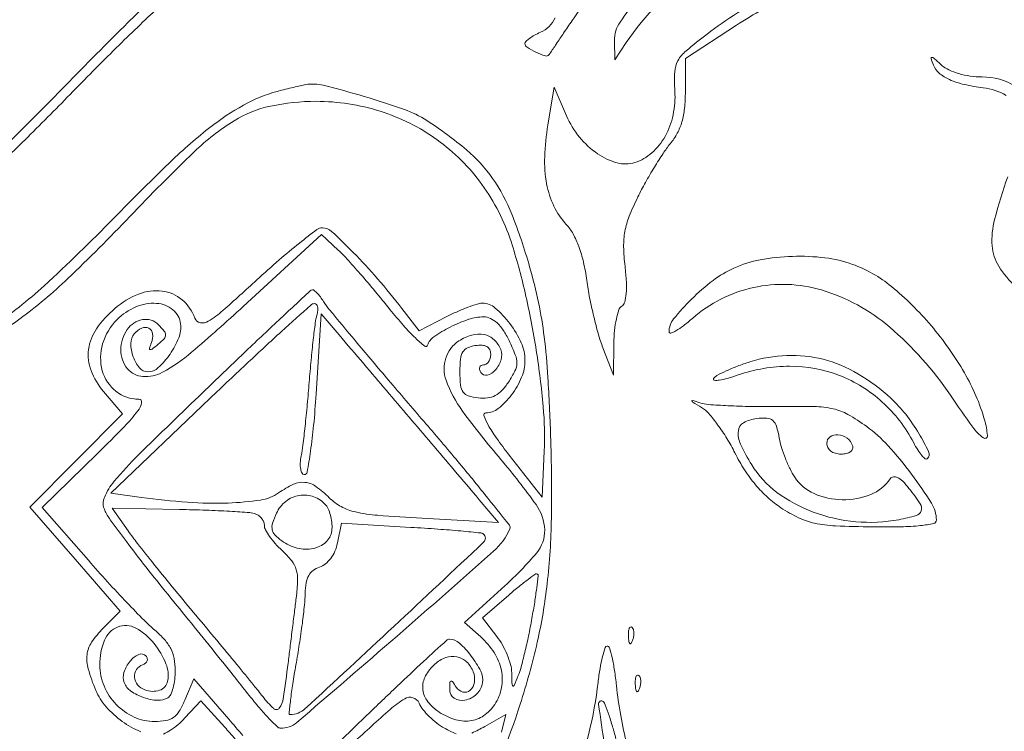
# Model space of a CAD drawing. Units: inches. Extents: x 2656 to 9931, y 1941 to 3068.
# Tile 37 of 46: x 2837 to 2847, y 2974 to 2981. Entities that reach past the tile are written whole.
import ezdxf

# ---------------------------------------------------------------- set-up
doc = ezdxf.new("R2010")
doc.units = ezdxf.units.IN
doc.layers.add('A-ANNO-DIMS', color=2, linetype='Continuous', lineweight=18)
doc.layers.add('A-ELEV-ORN', color=8, linetype='Continuous', lineweight=13)
doc.styles.get("Standard").update_dxf_attribs({"font": 'arial.ttf'})
doc.dimstyles.new('ISO-25', dxfattribs={"dimtxt": 6, "dimasz": 2.5, "dimexe": 1.25, "dimexo": 0.625, "dimtad": 1, "dimdec": 0, "dimlunit": 3, "dimtxsty": 'Standard', "dimcen": 2.5, "dimadec": 0, "dimazin": 0, "dimtfac": 1, "dimtdec": 0, "dimtmove": 0, "dimatfit": 3, "dimfxl": 1, "dimarcsym": 0})

# ---------------------------------------------------------------- blocks, each defined once
blk = doc.blocks.new('*D152')
at = {"layer": 'A-ANNO-DIMS', "color": 0, "lineweight": -2, "transparency": 16777216}
for p, q in [((2847.28, 2990.828), (2707.323, 2990.828)), ((2708.573, 2988.328), (2708.573, 2952.971)), ((2847.248, 2950.471), (2707.323, 2950.471))]:
    blk.add_line(p, q, dxfattribs=at)
at = {"layer": 'A-ANNO-DIMS', "color": 0, "transparency": 16777216}
for points in [[(2708.156, 2988.328), (2708.989, 2988.328), (2708.573, 2990.828)], [(2708.156, 2952.971), (2708.989, 2952.971), (2708.573, 2950.471)]]:
    blk.add_solid(points, dxfattribs=at)
at = {"layer": 'Defpoints', "color": 0, "transparency": 16777216}
for p in [(2847.905, 2990.828), (2708.573, 2950.471), (2847.873, 2950.471)]:
    blk.add_point(p, dxfattribs=at)
at = {"layer": 'A-ANNO-DIMS', "color": 0, "transparency": 16777216, "insert": (2704.843, 2970.649), "char_height": 6, "attachment_point": 5, "rotation": 90}
blk.add_mtext('3\'-4 1/2"', dxfattribs=at)
blk = doc.blocks.new('*D153')
at = {"layer": 'A-ANNO-DIMS', "color": 0, "lineweight": -2, "transparency": 16777216}
for p, q in [((2826.64, 2993.722), (2826.64, 2703.709)), ((2829.546, 2956.424), (2829.546, 2703.709)), ((2824.14, 2704.959), (2821.64, 2704.959)), ((2826.64, 2704.959), (2829.546, 2704.959)), ((2832.046, 2704.959), (2851.745, 2704.959))]:
    blk.add_line(p, q, dxfattribs=at)
at = {"layer": 'A-ANNO-DIMS', "color": 0, "transparency": 16777216}
for points in [[(2824.14, 2705.376), (2824.14, 2704.543), (2826.64, 2704.959)], [(2832.046, 2705.376), (2832.046, 2704.543), (2829.546, 2704.959)]]:
    blk.add_solid(points, dxfattribs=at)
at = {"layer": 'Defpoints', "color": 0, "transparency": 16777216}
for p in [(2826.64, 2994.347), (2829.546, 2957.049), (2829.546, 2704.959)]:
    blk.add_point(p, dxfattribs=at)
at = {"layer": 'A-ANNO-DIMS', "color": 0, "transparency": 16777216, "insert": (2843.145, 2708.65), "char_height": 6, "attachment_point": 5}
blk.add_mtext('0\'-3"', dxfattribs=at)
blk = doc.blocks.new('*D154')
at = {"layer": 'A-ANNO-DIMS', "color": 0, "lineweight": -2, "transparency": 16777216}
for p, q in [((2708.573, 2996.847), (2708.573, 2999.347)), ((2826.015, 2994.347), (2707.323, 2994.347)), ((2708.573, 2994.347), (2708.573, 2990.828)), ((2847.28, 2990.828), (2707.323, 2990.828)), ((2708.573, 2988.328), (2708.573, 2954.647))]:
    blk.add_line(p, q, dxfattribs=at)
at = {"layer": 'A-ANNO-DIMS', "color": 0, "transparency": 16777216}
for points in [[(2708.156, 2996.847), (2708.989, 2996.847), (2708.573, 2994.347)], [(2708.156, 2988.328), (2708.989, 2988.328), (2708.573, 2990.828)]]:
    blk.add_solid(points, dxfattribs=at)
at = {"layer": 'Defpoints', "color": 0, "transparency": 16777216}
for p in [(2826.64, 2994.347), (2708.573, 2990.828), (2847.905, 2990.828)]:
    blk.add_point(p, dxfattribs=at)
at = {"layer": 'A-ANNO-DIMS', "color": 0, "transparency": 16777216, "insert": (2704.843, 2970.237), "char_height": 6, "attachment_point": 5, "rotation": 90}
blk.add_mtext('0\'-3 1/2"', dxfattribs=at)

msp = doc.modelspace()

# ---------------------------------------------------------------- linework, layer by layer
at = {"layer": 'A-ELEV-ORN'}
for points in [[(2843.287, 2981.434, 0.03621), (2843.078, 2981.168, 0.154288), (2843.021, 2980.977), (2843.025, 2980.781), (2843.141, 2980.957, -0.10364), (2843.864, 2981.673, -0.058168)], [(2838.429, 2981.536, 0.015337), (2838.032, 2981.164, 0.003566), (2837.388, 2980.515, -0.006917), (2836.411, 2979.542, -0.058589)], [(2842.412, 2981.21, -0.182333), (2842.262, 2981.063, 0.022825), (2842.201, 2981.033, 0.031511), (2842.15, 2981.001, 0.032465), (2842.113, 2980.97, 0.205381), (2842.103, 2980.948, 0.258997), (2842.125, 2980.909, 0.02901), (2842.216, 2980.859, 0.028443), (2842.312, 2980.821, 0.331182), (2842.348, 2980.832, 0.005745), (2842.359, 2980.847, 0.000069), (2842.424, 2980.943, 0.000207), (2842.499, 2981.055, 0.000135), (2842.586, 2981.183, -0.032972), (2842.766, 2981.414, -0.024978)], [(2844.611, 2981.454, 0.041345), (2843.97, 2981.045, 0.012422), (2843.756, 2980.873, 0.08934), (2843.671, 2980.772, 0.116865), (2843.639, 2980.659, 0.027568), (2843.64, 2980.461, -0.06666), (2843.622, 2980.216, -0.076127), (2843.54, 2979.995, -0.083416), (2843.404, 2979.826, -0.105849), (2843.23, 2979.727, -0.146298), (2843.049, 2979.724, -0.081587), (2842.847, 2979.818, -0.071959), (2842.662, 2979.988, -0.069706), (2842.53, 2980.205), (2842.404, 2980.5), (2842.338, 2980.113, 0.033294), (2842.305, 2979.786, 0.054391), (2842.325, 2979.509, 0.06435), (2842.4, 2979.279, 0.078797), (2842.527, 2979.092, -0.063965), (2842.596, 2978.996, -0.036895), (2842.655, 2978.865, -0.031809), (2842.703, 2978.705, -0.02174), (2842.737, 2978.518, 0.014131), (2842.766, 2978.341, 0.010438), (2842.809, 2978.146, 0.010567), (2842.857, 2977.964, 0.02318), (2842.902, 2977.827), (2843.012, 2977.546), (2843.015, 2977.876, -0.021654), (2843.022, 2978.005, -0.028485), (2843.04, 2978.123, -0.02852), (2843.065, 2978.215, -0.175083), (2843.095, 2978.253, 0.191482), (2843.126, 2978.295, 0.044203), (2843.141, 2978.383, 0.034413), (2843.143, 2978.505, 0.016252), (2843.129, 2978.662, -0.024153), (2843.115, 2978.864, -0.051276), (2843.128, 2979.021, -0.049119), (2843.172, 2979.176, -0.020512), (2843.261, 2979.374, -0.011748), (2843.339, 2979.523, -0.009449), (2843.43, 2979.68, -0.009574), (2843.52, 2979.821, -0.023996), (2843.592, 2979.919, 0.047079), (2843.665, 2980.028, 0.051846), (2843.713, 2980.146, 0.045581), (2843.739, 2980.283, 0.025631), (2843.748, 2980.453), (2843.748, 2980.794), (2844.271, 2981.135, -0.0302), (2844.821, 2981.45, -0.01769)], [(2836.567, 2979.568, 0.006325), (2837.004, 2979.988, 0.004959), (2837.467, 2980.455, -0.005395), (2837.941, 2980.932, -0.007752), (2838.373, 2981.344, -0.006437)], [(2847.133, 2980.51, 0.135833), (2846.791, 2980.605, -0.034455), (2846.669, 2980.614, -0.035986), (2846.552, 2980.639, -0.038843), (2846.451, 2980.677, -0.074794), (2846.379, 2980.724, 0.003903), (2846.296, 2980.798, 0.174018), (2846.275, 2980.806, 0.52111), (2846.267, 2980.796, 0.011603), (2846.292, 2980.727, 0.127356), (2846.35, 2980.645, 0.067564), (2846.456, 2980.578, 0.051419), (2846.607, 2980.528, 0.027323), (2846.802, 2980.495, -0.106727), (2847.038, 2980.415, -0.193218)], [(2841.622, 2973.085, 0.033435), (2842.054, 2974.17, 0.022106), (2842.229, 2974.807, 0.027907), (2842.331, 2975.409, 0.024499), (2842.374, 2976.078, 0.01216), (2842.366, 2976.928, 0.005937), (2842.338, 2977.523, 0.016409), (2842.3, 2977.941, 0.021065), (2842.242, 2978.291, 0.017571), (2842.151, 2978.657, 0.023839), (2841.968, 2979.198, 0.059933), (2841.771, 2979.564, 0.064612), (2841.503, 2979.857, 0.031503), (2841.095, 2980.159, 0.05851), (2840.866, 2980.271, 0.013141), (2840.454, 2980.405, 0.01065), (2840.035, 2980.52, 0.1037), (2839.853, 2980.526, 0.014324), (2839.83, 2980.522, 0.001019), (2839.766, 2980.507, 0.001435), (2839.69, 2980.489, 0.001083), (2839.607, 2980.469, 0.059748), (2839.261, 2980.339, 0.043464), (2838.914, 2980.119, 0.028294), (2838.492, 2979.757, 0.008179), (2837.883, 2979.153, -0.013785), (2837.173, 2978.463, -0.04137), (2836.639, 2978.049, -0.055454)], [(2836.475, 2977.845, 0.04115), (2836.923, 2978.123, 0.031024), (2837.416, 2978.538, 0.011839), (2838.051, 2979.173, -0.010393), (2838.711, 2979.837, -0.053527), (2839.121, 2980.156, -0.085812), (2839.493, 2980.305, -0.05339), (2839.962, 2980.355, -0.075932), (2840.619, 2980.253, -0.079815), (2841.202, 2979.961, -0.080278), (2841.662, 2979.502, -0.07808), (2841.96, 2978.917, -0.022688), (2842.105, 2978.391, -0.016798), (2842.219, 2977.798, -0.017075), (2842.29, 2977.225, -0.033266), (2842.3, 2976.765), (2842.279, 2976.295), (2841.941, 2976.727, -0.011717), (2841.811, 2976.901, -0.0274), (2841.724, 2977.038, -0.040276), (2841.681, 2977.132, -0.520161), (2841.7, 2977.159, 0.169706), (2841.829, 2977.204, 0.064029), (2841.965, 2977.344, 0.061429), (2842.069, 2977.525, 0.099628), (2842.103, 2977.698, 0.106882), (2842.065, 2977.877, 0.054299), (2841.947, 2978.076, 0.054993), (2841.798, 2978.235, 0.178911), (2841.665, 2978.284, 0.077473), (2841.612, 2978.276, 0.013583), (2841.517, 2978.243, 0.014445), (2841.407, 2978.197, 0.012527), (2841.294, 2978.143), (2841.017, 2978.002), (2840.84, 2978.231, 0.013306), (2840.591, 2978.536, 0.016469), (2840.342, 2978.806, 0.011517), (2840.12, 2979.021, 0.188894), (2840.026, 2979.058, 0.16301), (2839.969, 2979.039, 0.006249), (2839.791, 2978.901, 0.01062), (2839.582, 2978.728, 0.007226), (2839.353, 2978.523, -0.003927), (2839.006, 2978.21, -0.043676), (2838.856, 2978.099, -0.190144), (2838.774, 2978.084, -0.259956), (2838.718, 2978.132, 0.129765), (2838.586, 2978.32, 0.145936), (2838.383, 2978.409, 0.124961), (2838.14, 2978.377, 0.082775), (2837.898, 2978.231, 0.064931), (2837.71, 2978.023, 0.11803), (2837.628, 2977.811, 0.127157), (2837.653, 2977.595, 0.082216), (2837.782, 2977.378), (2837.975, 2977.149), (2837.5, 2976.67), (2837.024, 2976.191), (2837.489, 2975.658), (2837.953, 2975.125), (2837.778, 2974.95, 0.047501), (2837.659, 2974.806, 0.119853), (2837.612, 2974.68, 0.100939), (2837.624, 2974.533, 0.027955), (2837.702, 2974.313, 0.082033), (2837.807, 2974.146, 0.055976), (2837.973, 2973.995, 0.057004), (2838.163, 2973.889, 0.09937)], [(2847.053, 2979.582, 0.019278), (2846.919, 2979.144, 0.083581), (2846.894, 2978.874, 0.121858), (2846.962, 2978.664, 0.063929), (2847.137, 2978.451, 0.026315)], [(2839.211, 2973.849, 0.001706), (2839.065, 2974.018), (2838.707, 2974.43), (2838.615, 2974.212, -0.036518), (2838.558, 2974.1, -0.103513), (2838.499, 2974.036, -0.109873), (2838.421, 2974.004, -0.044139), (2838.306, 2973.994, -0.107163), (2838.096, 2974.039, -0.093737), (2837.912, 2974.169, -0.092451), (2837.787, 2974.358, -0.100628), (2837.743, 2974.574, -0.093656), (2837.791, 2974.827, -0.208791), (2837.926, 2974.963, -0.2208), (2838.112, 2974.952, -0.102595), (2838.3, 2974.793, -0.067752), (2838.421, 2974.587, -0.148877), (2838.439, 2974.408, -0.271064), (2838.356, 2974.314, -0.172466), (2838.206, 2974.318, -0.12491), (2838.131, 2974.371, -0.154981), (2838.098, 2974.449, -0.174166), (2838.118, 2974.526, -0.158898), (2838.182, 2974.576, 0.082365), (2838.212, 2974.593, 0.13616), (2838.228, 2974.615, 0.15765), (2838.23, 2974.641, 0.121656), (2838.216, 2974.666, 0.318424), (2838.142, 2974.681, 0.119261), (2838.054, 2974.613, 0.092781), (2837.991, 2974.498, 0.171166), (2837.994, 2974.393, 0.150243), (2838.062, 2974.305, 0.068796), (2838.193, 2974.239, 0.068958), (2838.336, 2974.211, 0.154028), (2838.442, 2974.238, 0.152931), (2838.471, 2974.271, 0.038073), (2838.495, 2974.339, 0.03536), (2838.511, 2974.426, 0.029159), (2838.516, 2974.519, 0.047644), (2838.505, 2974.64, 0.069829), (2838.47, 2974.742, 0.065034), (2838.407, 2974.834, 0.035571), (2838.308, 2974.93, -0.022457), (2838.198, 2975.032, -0.005134), (2838.021, 2975.213, -0.0053), (2837.822, 2975.427, -0.00514), (2837.626, 2975.647), (2837.152, 2976.188), (2837.719, 2976.744, 0.005485), (2837.996, 2977.02, 0.030532), (2838.133, 2977.179, 0.10707), (2838.172, 2977.263, 0.481689), (2838.143, 2977.3, -0.168741), (2837.909, 2977.381, -0.160047), (2837.769, 2977.592, -0.140333), (2837.772, 2977.868, -0.124395), (2837.92, 2978.116, -0.095365), (2838.113, 2978.247, -0.118563), (2838.326, 2978.283, -0.155397), (2838.493, 2978.217, -0.195149), (2838.572, 2978.072, -0.125361), (2838.553, 2977.93, -0.054863), (2838.463, 2977.762, -0.055236), (2838.343, 2977.624, -0.189283), (2838.235, 2977.581, -0.223229), (2838.15, 2977.621, -0.088782), (2838.085, 2977.736, -0.084459), (2838.061, 2977.872, -0.175204), (2838.097, 2977.971, -0.111765), (2838.173, 2978.029, -0.231702), (2838.245, 2978.028, -0.248924), (2838.285, 2977.971, -0.121457), (2838.273, 2977.88, 0.015038), (2838.253, 2977.821, 0.435348), (2838.26, 2977.809, 0.22796), (2838.279, 2977.813, 0.007714), (2838.342, 2977.864, 0.030369), (2838.403, 2977.92, 0.191075), (2838.418, 2977.959, 0.174043), (2838.403, 2977.999, 0.024397), (2838.343, 2978.066, 0.248048), (2838.181, 2978.116, 0.196501), (2838.025, 2978.015, 0.150305), (2837.958, 2977.806, 0.177708), (2838.027, 2977.612, 0.207214), (2838.185, 2977.532, 0.139549), (2838.386, 2977.576, 0.053743), (2838.685, 2977.781, 0.008676), (2839.214, 2978.251), (2840.017, 2978.989), (2840.188, 2978.83, -0.020952), (2840.277, 2978.74, -0.00519), (2840.414, 2978.586, -0.005299), (2840.568, 2978.405, -0.00529), (2840.718, 2978.221, 0.011865), (2840.858, 2978.054, 0.022244), (2840.979, 2977.928, 0.022603), (2841.075, 2977.845, 0.520472), (2841.104, 2977.853, -0.163389), (2841.17, 2977.94, -0.033505), (2841.337, 2978.04, -0.035884), (2841.526, 2978.119, -0.08112), (2841.679, 2978.144, -0.109316), (2841.75, 2978.128, -0.078274), (2841.817, 2978.083, -0.061221), (2841.88, 2978.007, -0.033326), (2841.94, 2977.902, -0.017688), (2842.004, 2977.754, -0.097111), (2842.02, 2977.669, -0.113824), (2842, 2977.59, -0.028431), (2841.934, 2977.475, -0.041916), (2841.867, 2977.389, -0.085183), (2841.798, 2977.337, -0.09271), (2841.72, 2977.313, -0.057182), (2841.624, 2977.313, -0.046313), (2841.522, 2977.335, -0.165597), (2841.468, 2977.373, -0.12998), (2841.442, 2977.443, -0.024314), (2841.435, 2977.581, -0.025164), (2841.442, 2977.711, -0.108349), (2841.466, 2977.784, -0.155287), (2841.513, 2977.826, -0.070402), (2841.594, 2977.85, -0.046348), (2841.664, 2977.853, -0.116249), (2841.713, 2977.839, -0.157322), (2841.741, 2977.808, -0.110326), (2841.752, 2977.762, -0.065674), (2841.746, 2977.719, -0.083), (2841.73, 2977.684, -0.099141), (2841.706, 2977.66, -0.146526), (2841.677, 2977.651, 0.123549), (2841.653, 2977.645, 0.188168), (2841.639, 2977.629, 0.149887), (2841.638, 2977.604, 0.073526), (2841.65, 2977.574, 0.323078), (2841.717, 2977.547, 0.15707), (2841.799, 2977.597, 0.10622), (2841.858, 2977.704, 0.165993), (2841.854, 2977.809, 0.114288), (2841.786, 2977.91, 0.137455), (2841.684, 2977.963, 0.12038), (2841.559, 2977.958, 0.076057), (2841.425, 2977.897, 0.171637), (2841.291, 2977.721, 0.164234), (2841.294, 2977.495, 0.074473), (2841.464, 2977.176, 0.015793), (2841.856, 2976.681, -0.019559), (2842.217, 2976.218, -0.148597), (2842.305, 2975.959, -0.18523), (2842.223, 2975.724, -0.0338), (2841.898, 2975.387), (2841.482, 2975.011), (2841.649, 2974.862, -0.068545), (2841.787, 2974.7, -0.091238), (2841.861, 2974.52, -0.099477), (2841.862, 2974.339, -0.097525), (2841.793, 2974.169, -0.099545), (2841.679, 2974.053, -0.1212), (2841.536, 2974, -0.109868), (2841.374, 2974.018, -0.071304), (2841.205, 2974.103, -0.087768), (2841.097, 2974.211, -0.139844), (2841.055, 2974.334, -0.138306), (2841.083, 2974.461, -0.085038), (2841.179, 2974.582, -0.098996), (2841.29, 2974.649, -0.135105), (2841.405, 2974.657, -0.141194), (2841.505, 2974.605, -0.112222), (2841.573, 2974.504, -0.126558), (2841.585, 2974.398, -0.176252), (2841.541, 2974.314, -0.252155), (2841.467, 2974.296, -0.190975), (2841.398, 2974.346, 0.012851), (2841.36, 2974.403, 0.332859), (2841.344, 2974.408, 0.305494), (2841.333, 2974.394, 0.011688), (2841.331, 2974.323, 0.253566), (2841.378, 2974.233, 0.199334), (2841.488, 2974.212, 0.143874), (2841.609, 2974.276, 0.165626), (2841.668, 2974.392, 0.152851), (2841.649, 2974.51, 0.046058), (2841.552, 2974.665, 0.045522), (2841.43, 2974.799, 0.187028), (2841.329, 2974.838, 0.187242), (2841.299, 2974.826, 0.000977), (2841.062, 2974.609, 0.004125), (2840.794, 2974.357, 0.002582), (2840.483, 2974.058), (2839.681, 2973.279)], [(2843.15, 2973.753, -0.035809), (2843.041, 2974.363, 0.011612), (2843.021, 2974.518, 0.018786), (2842.996, 2974.649, 0.013281), (2842.969, 2974.751, 0.334222), (2842.947, 2974.767, 0.326018), (2842.925, 2974.752, 0.015343), (2842.899, 2974.659, 0.020323), (2842.873, 2974.539, 0.012637), (2842.853, 2974.397, -0.062714), (2842.597, 2973.361, -0.053881)], [(2840.342, 2973.776, -0.00338), (2840.721, 2974.118, -0.04635), (2840.87, 2974.228, -0.212535), (2840.954, 2974.238, -0.217548), (2841.017, 2974.182, 0.062816), (2841.056, 2974.117, 0.030913), (2841.121, 2974.045, 0.030087), (2841.199, 2973.977, 0.038409), (2841.278, 2973.925, 0.028926), (2841.396, 2973.869, 0.107992)], [(2838.395, 2973.865, 0.034437), (2838.468, 2973.905, 0.032541), (2838.546, 2973.962, 0.031042), (2838.616, 2974.03), (2838.78, 2974.206), (2839.024, 2973.936, -0.00618), (2839.13, 2973.816, -0.004408)], [(2841.559, 2973.875, 0.02151), (2841.69, 2973.942), (2841.908, 2974.067), (2841.863, 2973.884, -0.047953)]]:
    msp.add_lwpolyline(points, format="xyb", dxfattribs=at)
for points in [[(2844.246, 2978.644, 0.055126), (2844.033, 2978.518, 0.032593), (2843.81, 2978.325, 0.029406), (2843.627, 2978.123, 0.170686), (2843.58, 2977.99, 0.507324), (2843.598, 2977.978, 0.054143), (2843.651, 2978.001, 0.033257), (2843.728, 2978.053, 0.016009), (2843.821, 2978.129, -0.126434), (2844.445, 2978.445, -0.127367), (2845.143, 2978.42, -0.105379), (2845.843, 2978.039, -0.066514), (2846.465, 2977.342, 0.006862), (2846.694, 2977.014, 0.080044), (2846.804, 2976.903, 0.637279), (2846.845, 2976.926, 0.05218), (2846.816, 2977.087, 0.062327), (2846.609, 2977.571, 0.043802), (2846.267, 2978.056, 0.044744), (2845.86, 2978.456, 0.08537), (2845.463, 2978.683, 0.056881), (2845.179, 2978.75, 0.038039), (2844.846, 2978.765, 0.038215), (2844.516, 2978.73, 0.060608)], [(2838.802, 2977.371, 0.002251), (2838.14, 2976.729, 0.025034), (2837.891, 2976.458, 0.074037), (2837.79, 2976.293, 0.213712), (2837.793, 2976.162, 0.045898), (2837.851, 2976.064, 0.004408), (2838.016, 2975.84, 0.005583), (2838.218, 2975.576, 0.004379), (2838.443, 2975.295, -0.000739), (2838.682, 2975.001, -0.000694), (2838.924, 2974.701, -0.00069), (2839.139, 2974.434, -0.002399), (2839.276, 2974.261, 0.009705), (2839.38, 2974.133, 0.014096), (2839.477, 2974.026, 0.009596), (2839.561, 2973.941, 0.182005), (2839.594, 2973.926, 0.192236), (2839.763, 2973.984, 0.001742), (2840.791, 2974.87, 0.002684), (2841.782, 2975.741, 0.109878), (2841.949, 2975.971, 0.276531), (2841.944, 2976.007, 0.001195), (2841.691, 2976.323, 0.005179), (2841.397, 2976.683, 0.003186), (2841.042, 2977.1, -0.001401), (2840.681, 2977.522, -0.002019), (2840.364, 2977.898, -0.001051), (2840.098, 2978.218, -0.03251), (2840.037, 2978.302, 0.020668), (2840.005, 2978.349, 0.028592), (2839.972, 2978.388, 0.028245), (2839.942, 2978.416, 0.202446), (2839.924, 2978.421, 0.164032), (2839.899, 2978.41, 0.000327), (2839.579, 2978.111, 0.00224), (2839.221, 2977.773, 0.001381)], [(2839.969, 2978.161, 0.035549), (2839.953, 2978.084, 0.004113), (2839.931, 2977.909, 0.004933), (2839.91, 2977.7, 0.004008), (2839.89, 2977.475, -0.003598), (2839.871, 2977.246, -0.003827), (2839.848, 2977.021, -0.003645), (2839.826, 2976.828, -0.017645), (2839.809, 2976.719, 0.03281), (2839.799, 2976.645, 0.055472), (2839.803, 2976.583, 0.079731), (2839.817, 2976.54, 0.280048), (2839.84, 2976.526, 0.364768), (2839.87, 2976.551, 0.006646), (2839.904, 2976.767, 0.012967), (2839.936, 2977.032, 0.007717), (2839.961, 2977.35), (2840.012, 2978.175), (2840.196, 2977.96, -0.000676), (2840.45, 2977.662, -0.000127), (2840.914, 2977.117, -0.000128), (2841.377, 2976.572, -0.000658), (2841.634, 2976.269), (2841.832, 2976.034), (2841.047, 2976.078, -0.005429), (2840.592, 2976.109, -0.034904), (2840.365, 2976.143, -0.069359), (2840.219, 2976.198, -0.072692), (2840.096, 2976.289, 0.042326), (2839.959, 2976.405, 0.131102), (2839.846, 2976.447, 0.133074), (2839.729, 2976.427, 0.044175), (2839.577, 2976.339, -0.116822), (2839.391, 2976.265, -0.028124), (2839.059, 2976.235, -0.025614), (2838.643, 2976.243, -0.017115), (2838.169, 2976.292), (2837.856, 2976.335), (2838.872, 2977.307, -0.002498), (2839.266, 2977.679, -0.003976), (2839.606, 2977.994, -0.00097), (2839.906, 2978.265, -0.171827), (2839.945, 2978.281, -0.245897), (2839.964, 2978.272, -0.117644), (2839.976, 2978.247, -0.074451), (2839.978, 2978.208, -0.041352)], [(2844.41, 2977.683, 0.013747), (2844.281, 2977.638, 0.017821), (2844.165, 2977.589, 0.015655), (2844.072, 2977.543, 0.131684), (2844.038, 2977.512, 0.541186), (2844.046, 2977.494, 0.070976), (2844.095, 2977.495, 0.034041), (2844.18, 2977.513, 0.014954), (2844.29, 2977.548, -0.0851), (2844.817, 2977.638, -0.092256), (2845.328, 2977.543, -0.092941), (2845.767, 2977.271, -0.08785), (2846.089, 2976.853, 0.019883), (2846.131, 2976.779, 0.035518), (2846.173, 2976.723, 0.044453), (2846.208, 2976.688, 0.386642), (2846.228, 2976.689, 0.31585), (2846.241, 2976.763, 0.025842), (2846.143, 2976.947, 0.031419), (2846.007, 2977.145, 0.038824), (2845.855, 2977.309, 0.054014), (2845.517, 2977.561, 0.069968), (2845.16, 2977.709, 0.073126), (2844.79, 2977.748, 0.066506)], [(2843.914, 2977.214, -0.077083), (2843.987, 2977.154, -0.021908), (2844.079, 2977.038, -0.021512), (2844.174, 2976.897, -0.021261), (2844.256, 2976.748, 0.027573), (2844.355, 2976.575, 0.031394), (2844.467, 2976.422, 0.033051), (2844.592, 2976.292, 0.038975), (2844.727, 2976.187, 0.034341), (2844.909, 2976.084, 0.060401), (2845.073, 2976.028, 0.04034), (2845.286, 2976.001, 0.008154), (2845.668, 2975.99, 0.007564), (2845.96, 2975.991, 0.022257), (2846.16, 2976.004, 0.025839), (2846.294, 2976.025, 0.358656), (2846.322, 2976.061, 0.136318), (2846.272, 2976.232, 0.020432), (2846.067, 2976.53, 0.024075), (2845.825, 2976.824, 0.051771), (2845.607, 2977.019, 0.028184), (2845.415, 2977.143, 0.07446), (2845.263, 2977.201, 0.04988), (2845.068, 2977.224, 0.007562), (2844.675, 2977.225, -0.006906), (2844.421, 2977.225, -0.008509), (2844.184, 2977.233, -0.007223), (2843.985, 2977.245, -0.059977), (2843.897, 2977.263, 0.004444), (2843.818, 2977.288, 0.61372), (2843.813, 2977.283, 0.173814), (2843.823, 2977.27, 0.002263)], [(2844.869, 2976.5, 0.144478), (2845.068, 2976.331, 0.100358), (2845.357, 2976.268, 0.100739), (2845.648, 2976.322, 0.14681), (2845.849, 2976.484, -0.209804), (2845.882, 2976.504, -0.15493), (2845.924, 2976.497, -0.080271), (2845.977, 2976.458, -0.027211), (2846.041, 2976.385, -0.01924), (2846.156, 2976.227, -0.230516), (2846.166, 2976.155, -0.250068), (2846.115, 2976.106, -0.022372), (2845.936, 2976.064, -0.069095), (2845.496, 2976.043, -0.0666), (2845.06, 2976.142, -0.070186), (2844.687, 2976.344, -0.095397), (2844.428, 2976.626, -0.029261), (2844.314, 2976.838, -0.135726), (2844.291, 2976.974, -0.240815), (2844.345, 2977.058, -0.102338), (2844.477, 2977.101, -0.040999), (2844.584, 2977.105, -0.166081), (2844.644, 2977.081, -0.143489), (2844.682, 2977.023, -0.028057), (2844.711, 2976.901, 0.029707), (2844.735, 2976.803, 0.01874), (2844.774, 2976.692, 0.018806), (2844.821, 2976.584, 0.032563)], [(2845.462, 2976.825, -0.158297), (2845.462, 2976.79, -0.156475), (2845.442, 2976.761, -0.107922), (2845.401, 2976.743, -0.053387), (2845.345, 2976.737, -0.066422), (2845.286, 2976.745, -0.09567), (2845.239, 2976.768, -0.111791), (2845.209, 2976.803, -0.12024), (2845.198, 2976.848, -0.245384), (2845.232, 2976.913, -0.175333), (2845.313, 2976.935, -0.13487), (2845.406, 2976.9, -0.158083)], [(2840.061, 2976.213, -0.074494), (2840.091, 2976.163, -0.041702), (2840.113, 2976.094, -0.040508), (2840.124, 2976.019, -0.051913), (2840.122, 2975.949, -0.17409), (2840.06, 2975.833, -0.136645), (2839.932, 2975.768, -0.112475), (2839.767, 2975.772, -0.095455), (2839.609, 2975.847, -0.042616), (2839.538, 2975.909, -0.146206), (2839.511, 2975.962, -0.126282), (2839.515, 2976.027, -0.02836), (2839.555, 2976.131, -0.121466), (2839.651, 2976.252, -0.12543), (2839.791, 2976.313, -0.128945), (2839.939, 2976.299, -0.132209)], [(2839.343, 2976.122, -0.077766), (2839.376, 2976.103, -0.065213), (2839.405, 2976.073, -0.066878), (2839.424, 2976.038, -0.092274), (2839.431, 2976.003, 0.127866), (2839.442, 2975.959, 0.027611), (2839.484, 2975.892, 0.027111), (2839.543, 2975.818, 0.023013), (2839.613, 2975.747, -0.036457), (2839.711, 2975.642, -0.097185), (2839.758, 2975.551, -0.081745), (2839.771, 2975.441, -0.020832), (2839.757, 2975.26, 0.000041), (2839.739, 2975.113, 0.000022), (2839.716, 2974.933, 0.000022), (2839.694, 2974.749, 0.000035), (2839.674, 2974.592, -0.005654), (2839.625, 2974.228, -0.126601), (2839.584, 2974.131, -0.445429), (2839.526, 2974.126, -0.040097), (2839.414, 2974.249, 0.006784), (2839.323, 2974.364, 0.001195), (2839.149, 2974.578, 0.001294), (2838.943, 2974.827, 0.001163), (2838.728, 2975.084, -0.002519), (2838.513, 2975.343, -0.002691), (2838.305, 2975.599, -0.002553), (2838.129, 2975.821, -0.012575), (2838.033, 2975.949), (2837.869, 2976.181), (2838.562, 2976.169, -0.004273), (2838.834, 2976.161, -0.005935), (2839.077, 2976.15, -0.003793), (2839.281, 2976.136, -0.072698)], [(2841.677, 2975.917, -0.442629), (2841.679, 2975.833, -0.001207), (2840.758, 2974.969, -0.001729), (2839.847, 2974.124, -0.188316), (2839.694, 2974.064, -0.444287), (2839.684, 2974.076, -0.003686), (2839.699, 2974.214, -0.009553), (2839.721, 2974.379, -0.005648), (2839.754, 2974.574, 0.006128), (2839.789, 2974.786, 0.005974), (2839.82, 2975, 0.005903), (2839.842, 2975.189, 0.022148), (2839.849, 2975.308, -0.036526), (2839.859, 2975.415, -0.084616), (2839.885, 2975.491, -0.106749), (2839.93, 2975.543, -0.084665), (2839.996, 2975.577, 0.093746), (2840.057, 2975.61, 0.06268), (2840.111, 2975.667, 0.057495), (2840.154, 2975.741, 0.053064), (2840.18, 2975.825), (2840.221, 2976.027), (2840.933, 2975.985, -0.003298), (2841.209, 2975.967, -0.005138), (2841.446, 2975.948, -0.001705), (2841.65, 2975.928, -0.1562)], [(2842.174, 2975.052, -0.006817), (2842.14, 2974.874, -0.007069), (2842.101, 2974.7, -0.006851), (2842.063, 2974.551, -0.030171), (2842.034, 2974.464, -0.003631), (2841.992, 2974.362, -0.422307), (2841.98, 2974.358, -0.2851), (2841.971, 2974.371, -0.002646), (2841.967, 2974.494, 0.060604), (2841.955, 2974.578, 0.030764), (2841.92, 2974.68, 0.030031), (2841.871, 2974.781, 0.039285), (2841.814, 2974.867), (2841.666, 2975.056), (2841.937, 2975.291, -0.007862), (2842.043, 2975.38, -0.012888), (2842.136, 2975.452, -0.006508), (2842.214, 2975.508, -0.354903), (2842.231, 2975.506, -0.234956), (2842.238, 2975.487, -0.003368), (2842.223, 2975.364, -0.00847), (2842.203, 2975.219, -0.005383)], [(2843.164, 2974.867, 0.018894), (2843.168, 2974.815, 0.168741), (2843.178, 2974.794, 0.470617), (2843.191, 2974.795, 0.054073), (2843.207, 2974.825, 0.051402), (2843.217, 2974.863, 0.05415), (2843.22, 2974.902, 0.060344), (2843.215, 2974.936, 0.126455), (2843.201, 2974.959, 0.296942), (2843.186, 2974.963, 0.208169), (2843.173, 2974.95, 0.077125), (2843.165, 2974.916, 0.028489)], [(2843.234, 2974.375, 0.018894), (2843.239, 2974.322, 0.168741), (2843.248, 2974.302, 0.470617), (2843.261, 2974.303, 0.054073), (2843.277, 2974.332, 0.051402), (2843.288, 2974.371, 0.05415), (2843.29, 2974.41, 0.060344), (2843.285, 2974.444, 0.126455), (2843.271, 2974.467, 0.296942), (2843.256, 2974.47, 0.208169), (2843.243, 2974.458, 0.077125), (2843.235, 2974.424, 0.028489)], [(2843.046, 2973.776, -0.013205), (2843.086, 2973.598, -0.006854), (2843.127, 2973.373, -0.00681), (2843.163, 2973.142, -0.010294), (2843.187, 2972.939, 0.000202), (2843.207, 2972.741, 0.000153), (2843.229, 2972.523, 0.000154), (2843.25, 2972.318, 0.000358), (2843.265, 2972.165, -0.001534), (2843.285, 2971.967, -0.110402), (2843.281, 2971.935, -0.7056), (2843.27, 2971.935, -0.004671), (2843.227, 2972.06, -0.036376), (2843.117, 2972.496, -0.006701), (2842.982, 2973.315, -0.002798), (2842.858, 2974.173, -0.711672), (2842.906, 2974.198, -0.114458), (2842.927, 2974.165, -0.007415), (2842.965, 2974.057, -0.010497), (2843.006, 2973.924, -0.007618)]]:
    msp.add_lwpolyline(points, format="xyb", close=True, dxfattribs=at)

# ---------------------------------------------------------------- dimensions: what is measured, and where the dimension line sits
at = {"layer": 'A-ANNO-DIMS'}
for base, p1, p2, picture, middle in [((2708.573, 2990.828), (2826.64, 2994.347), (2847.905, 2990.828), '*D154', (2704.843, 2970.237)), ((2708.573, 2950.471), (2847.905, 2990.828), (2847.873, 2950.471), '*D152', (2704.843, 2970.649))]:
    dim = msp.add_linear_dim(base=base, p1=p1, p2=p2, angle=90, dimstyle='ISO-25', override={"dimdec": 1, "dimlfac": 1, "dimrnd": 0, "dimzin": 1, "dimdsep": 46, "dimlunit": 4, "dimfrac": 2}, dxfattribs=at)
    dim.commit()
    dim.dimension.update_dxf_attribs({"geometry": picture, "text_midpoint": middle})
dim = msp.add_linear_dim(base=(2829.546, 2704.959), p1=(2826.64, 2994.347), p2=(2829.546, 2957.049), dimstyle='ISO-25', override={"dimdec": 1, "dimlfac": 1, "dimrnd": 0, "dimzin": 1, "dimdsep": 46, "dimlunit": 4, "dimfrac": 2}, dxfattribs=at)
dim.commit()
dim.dimension.update_dxf_attribs({"geometry": '*D153', "text_midpoint": (2843.145, 2708.65)})

doc.saveas('drawing.dxf')
